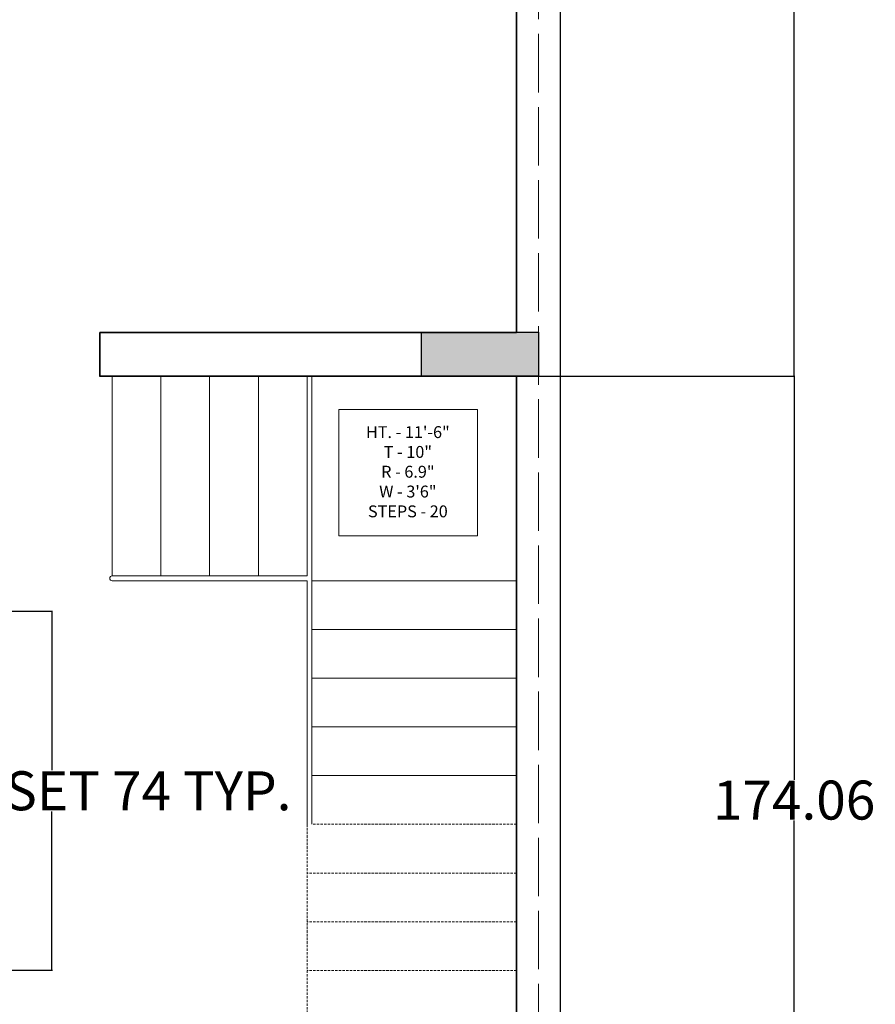
# Model space of a CAD drawing. Units: inches. Extents: x -48 to 50072, y 0 to 21068.
# Tile 70 of 75: x 1188 to 1363, y 803 to 1005. Entities that reach past the tile are written whole.
import ezdxf

# ---------------------------------------------------------------- set-up
doc = ezdxf.new("R2010")
doc.units = ezdxf.units.IN
doc.header["$MEASUREMENT"] = 0
doc.linetypes.add('ACAD_ISO02W100', pattern=[15, 12, -3])
doc.linetypes.add('DASHED', pattern=[0.75, 0.5, -0.25])
for name, color, linetype, lineweight in [('A-ANNO-DIMS', 2, 'Continuous', 18), ('A-ANNO-TEXT', 7, 'Continuous', 18), ('A-COLS', 1, 'Continuous', 35), ('A-FLOR-STRS', 7, 'Continuous', 18), ('A-FLOR-STRS-HIDN', 8, 'DASHED', 13), ('A-WALL', 7, 'Continuous', 35), ('C-PROP', 7, 'Continuous', 25), ('C-PROP-REF', 32, 'ACAD_ISO02W100', 13)]:
    doc.layers.add(name, color=color, linetype=linetype, lineweight=lineweight)
doc.styles.get("Standard").update_dxf_attribs({"font": 'arial.ttf'})
doc.dimstyles.get("Standard").update_dxf_attribs({"dimtxt": 8, "dimasz": 0.18, "dimexe": 0.18, "dimexo": 0.0625, "dimgap": 0.09, "dimtad": 0, "dimtih": 1, "dimtoh": 1, "dimdec": 1, "dimzin": 0, "dimdsep": 46, "dimlunit": 4, "dimtxsty": 'Standard', "dimblk": 'ARCHTICK', "dimcen": 0.09, "dimadec": 0, "dimazin": 0, "dimtfac": 1, "dimtdec": 1, "dimtofl": 0, "dimtmove": 0, "dimatfit": 3, "dimldrblk": 'ARCHTICK', "dimfxl": 1, "dimtolj": 1, "dimtzin": 0, "dimarcsym": 0})

# ---------------------------------------------------------------- blocks, each defined once
blk = doc.blocks.new('bnniku')
at = {"layer": 'Defpoints'}
h = blk.add_hatch(color=256, dxfattribs=at)
h.dxf.hatch_style = 1
h.paths.add_polyline_path([(767.55, 1114.04), (758.55, 1114.04), (758.55, 1090.04), (767.55, 1090.04)])
for p, q in [((758.55, 1114.04), (767.55, 1114.04)), ((758.55, 1090.04), (758.55, 1114.04)), ((767.55, 1114.04), (767.55, 1090.04)), ((767.55, 1090.04), (758.55, 1090.04))]:
    blk.add_line(p, q, dxfattribs=at)
blk = doc.blocks.new('_ArchTick')
at = {"color": 0, "linetype": 'ByBlock', "const_width": 0.15}
blk.add_lwpolyline([(-0.5, -0.5), (0.5, 0.5)], dxfattribs=at)
blk = doc.blocks.new('*D78')
at = {"layer": 'A-ANNO-DIMS', "color": 0, "lineweight": -2, "transparency": 16777216}
for p, q in [((1183.37, 883.26), (1194.54, 883.26)), ((1194.36, 883.26), (1194.36, 850.64)), ((1194.36, 809.56), (1194.36, 842.18)), ((1183.37, 809.56), (1194.54, 809.56))]:
    blk.add_line(p, q, dxfattribs=at)
at = {"layer": 'Defpoints', "color": 0, "transparency": 16777216}
for p in [(1183.3, 883.26), (1183.3, 809.56), (1194.36, 809.56)]:
    blk.add_point(p, dxfattribs=at)
at = {"layer": 'A-ANNO-DIMS', "color": 0, "lineweight": -2, "transparency": 16777216, "xscale": 0.18, "yscale": 0.18, "zscale": 0.18}
for p, rotation in [((1194.36, 883.26), 90), ((1194.36, 809.56), 270)]:
    blk.add_blockref('_ArchTick', p, dxfattribs=dict(at, rotation=rotation))
at = {"layer": 'A-ANNO-DIMS', "color": 0, "transparency": 16777216, "insert": (1194.36, 846.41), "char_height": 8, "attachment_point": 5}
blk.add_mtext('\\A1;DINING SET 74 TYP.', dxfattribs=at)
blk = doc.blocks.new('*D133')
at = {"layer": 'A-ANNO-DIMS', "color": 0, "lineweight": -2, "transparency": 16777216}
for p, q in [((1294.32, 1105.46), (1346.89, 1105.46)), ((1346.71, 1105.46), (1346.71, 1022.67)), ((1346.71, 931.53), (1346.71, 1014.32)), ((1294.32, 931.53), (1346.89, 931.53))]:
    blk.add_line(p, q, dxfattribs=at)
at = {"layer": 'Defpoints', "color": 0, "transparency": 16777216}
for p in [(1294.26, 1105.46), (1294.26, 931.53), (1346.71, 931.53)]:
    blk.add_point(p, dxfattribs=at)
at = {"layer": 'A-ANNO-DIMS', "color": 0, "lineweight": -2, "transparency": 16777216, "xscale": 0.18, "yscale": 0.18, "zscale": 0.18}
for p, rotation in [((1346.71, 1105.46), 90), ((1346.71, 931.53), 270)]:
    blk.add_blockref('_ArchTick', p, dxfattribs=dict(at, rotation=rotation))
at = {"layer": 'A-ANNO-DIMS', "color": 0, "transparency": 16777216, "insert": (1346.71, 1018.5), "char_height": 8, "attachment_point": 5}
blk.add_mtext('\\A1;173.94', dxfattribs=at)
blk = doc.blocks.new('*D134')
at = {"layer": 'A-ANNO-DIMS', "color": 0, "lineweight": -2, "transparency": 16777216}
for p, q in [((1294.32, 931.53), (1346.89, 931.53)), ((1346.71, 931.53), (1346.71, 848.67)), ((1346.71, 757.46), (1346.71, 840.32)), ((1294.32, 757.46), (1346.89, 757.46))]:
    blk.add_line(p, q, dxfattribs=at)
at = {"layer": 'Defpoints', "color": 0, "transparency": 16777216}
for p in [(1294.26, 931.53), (1294.26, 757.46), (1346.71, 757.46)]:
    blk.add_point(p, dxfattribs=at)
at = {"layer": 'A-ANNO-DIMS', "color": 0, "lineweight": -2, "transparency": 16777216, "xscale": 0.18, "yscale": 0.18, "zscale": 0.18}
for p, rotation in [((1346.71, 931.53), 90), ((1346.71, 757.46), 270)]:
    blk.add_blockref('_ArchTick', p, dxfattribs=dict(at, rotation=rotation))
at = {"layer": 'A-ANNO-DIMS', "color": 0, "transparency": 16777216, "insert": (1346.71, 844.5), "char_height": 8, "attachment_point": 5}
blk.add_mtext('\\A1;174.06', dxfattribs=at)

msp = doc.modelspace()

# ---------------------------------------------------------------- linework, layer by layer
at = {"layer": 'A-ANNO-TEXT'}
msp.add_lwpolyline([(1253.251, 924.677), (1281.708, 924.677), (1281.708, 898.759), (1253.251, 898.759)], close=True, dxfattribs=at)
at = {"layer": 'A-FLOR-STRS'}
for p, q in [((1206.761, 890.527), (1206.761, 931.527)), ((1216.761, 890.527), (1216.761, 931.527)), ((1226.761, 890.527), (1226.761, 931.527)), ((1236.761, 890.527), (1236.761, 931.527)), ((1246.761, 890.527), (1246.761, 931.527)), ((1247.761, 839.527), (1247.761, 931.527)), ((1246.761, 890.527), (1206.761, 890.527)), ((1246.761, 889.527), (1206.761, 889.527)), ((1246.761, 839.527), (1246.761, 889.527)), ((1289.761, 889.527), (1247.761, 889.527)), ((1289.761, 879.527), (1247.761, 879.527)), ((1289.761, 869.527), (1247.761, 869.527)), ((1289.761, 859.527), (1247.761, 859.527)), ((1289.761, 849.527), (1247.761, 849.527))]:
    msp.add_line(p, q, dxfattribs=at)
msp.add_arc((1206.761, 890.027), 0.5, 90, 270, dxfattribs=at)
at = {"layer": 'A-FLOR-STRS-HIDN'}
for p, q in [((1246.761, 839.527), (1246.761, 757.527)), ((1289.761, 839.527), (1247.761, 839.527)), ((1289.761, 829.527), (1246.761, 829.527)), ((1289.761, 819.527), (1246.761, 819.527)), ((1289.761, 809.527), (1246.761, 809.527))]:
    msp.add_line(p, q, dxfattribs=at)
at = {"layer": 'A-WALL'}
for p, q in [((1289.761, 940.464), (1289.761, 1096.464)), ((1204.261, 931.464), (1204.261, 940.464)), ((1289.761, 940.464), (1204.261, 940.464)), ((1294.261, 931.527), (1204.261, 931.527)), ((1289.761, 757.464), (1289.761, 931.527))]:
    msp.add_line(p, q, dxfattribs=at)
at = {"layer": 'C-PROP'}
msp.add_line((1298.761, 284.764), (1298.761, 1241.464), dxfattribs=at)
at = {"layer": 'C-PROP-REF'}
msp.add_line((1294.261, 284.764), (1294.261, 1236.964), dxfattribs=at)

# ---------------------------------------------------------------- block references
at = {"layer": 'A-COLS', "rotation": 270}
msp.add_blockref('bnniku', (180.224, 1699.079), dxfattribs=at)

# ---------------------------------------------------------------- texts
at = {"layer": 'A-ANNO-TEXT', "insert": (1247.859, 921.253), "char_height": 2.4397, "attachment_point": 1}
msp.add_mtext_dynamic_manual_height_columns('\\pxqc;HT. - 11\'-6"^JT - 10"^JR - 6.9"^JW - 3\'6"^JSTEPS - 20', width=39.17224, gutter_width=12.199, heights=[0], dxfattribs=at)

# ---------------------------------------------------------------- dimensions: what is measured, and where the dimension line sits
at = {"layer": 'A-ANNO-DIMS'}
for base, p1, p2, picture, middle in [((1346.711, 931.527), (1294.261, 1105.464), (1294.261, 931.527), '*D133', (1346.711, 1018.496)), ((1346.711, 757.464), (1294.261, 931.527), (1294.261, 757.464), '*D134', (1346.711, 844.496))]:
    dim = msp.add_linear_dim(base=base, p1=p1, p2=p2, angle=90, dimstyle='Standard', override={"dimdec": 2, "dimlfac": 1, "dimrnd": 0, "dimzin": 0, "dimdsep": 46, "dimlunit": 2}, dxfattribs=at)
    dim.commit()
    dim.dimension.update_dxf_attribs({"geometry": picture, "text_midpoint": middle})
dim = msp.add_linear_dim(base=(1194.358, 809.562), p1=(1183.303, 883.261), p2=(1183.303, 809.562), angle=270, text='DINING SET <> TYP.', dimstyle='Standard', override={"dimdec": 0, "dimlfac": 1, "dimrnd": 0, "dimzin": 0, "dimdsep": 46, "dimlunit": 2}, dxfattribs=at)
dim.commit()
dim.dimension.update_dxf_attribs({"geometry": '*D78', "text_midpoint": (1194.358, 846.411)})

doc.saveas('drawing.dxf')
